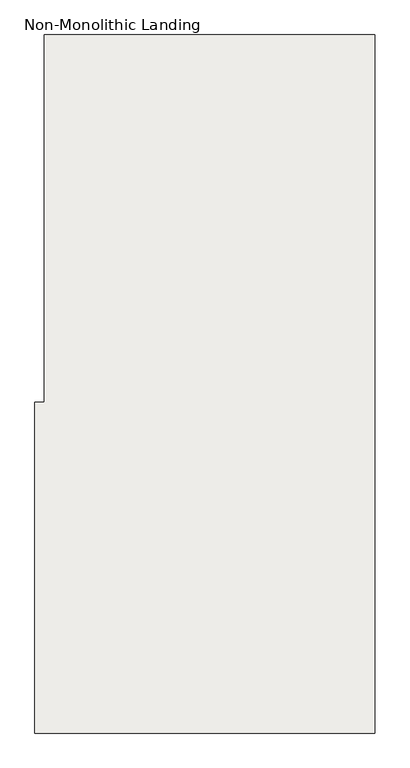
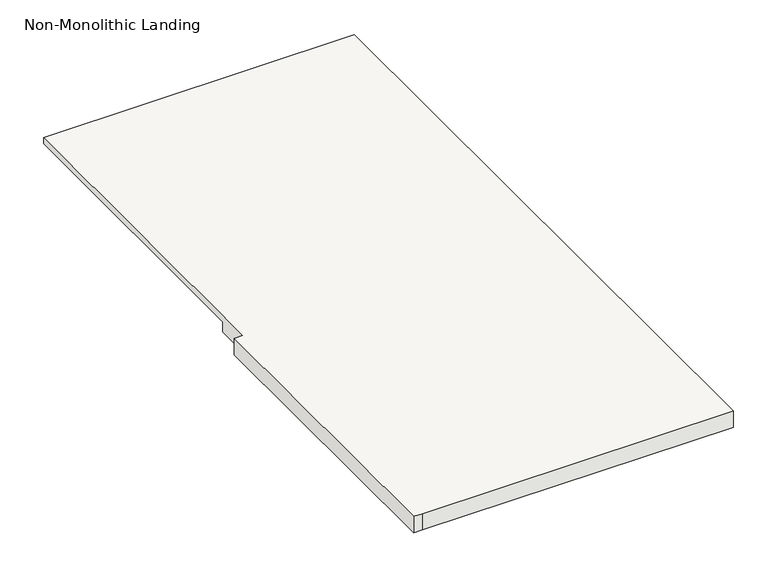
"""IFC4 building model written with IfcOpenShell, lengths in millimetres: slab geometry, Non-Monolithic Landing."""

from ifc_helpers import new_model, si_unit, origin, place, context, project, spatial, faceted_brep, source, transform, mapped, element, save


def non_monolithic_landing_f056e2ed(model_context):
    return source(origin(), model_context, "Body", "Brep", [
        faceted_brep([(923.4845537, -3822.9544725, 20783.55), (948.8845537, -3822.9544725, 20758.15), (948.8845537, -4737.3544725, 20758.15), (923.4845537, -4737.3544725, 20783.55), (923.4845537, -4838.9544725, 20802.6), (898.0845537, -4838.9544725, 20802.6), (898.0845537, -5753.3544725, 20802.6), (923.4845537, -5753.3544725, 20802.6), (1837.8845537, -5753.3544725, 20802.6), (1837.8845537, -3822.9544725, 20802.6), (923.4845537, -3822.9544725, 20802.6), (948.8845537, -4737.3544725, 20751.8), (948.8845537, -3822.9544725, 20751.8), (1837.8845537, -3822.9544725, 20751.8), (1837.8845537, -5753.3544725, 20751.8), (923.4845537, -5753.3544725, 20751.8), (898.0845537, -5753.3544725, 20751.8), (898.0845537, -4838.9544725, 20751.8), (923.4845537, -4838.9544725, 20751.8), (923.4845537, -4737.3544725, 20751.8)], [[[0, 1, 2, 3]], [[4, 5, 6, 7, 8, 9, 10]], [[11, 12, 13, 14, 15, 16, 17, 18, 19]], [[12, 11, 2, 1]], [[11, 19, 3, 2]], [[4, 10, 0, 3, 19, 18]], [[5, 4, 18, 17]], [[6, 5, 17, 16]], [[7, 6, 16, 15]], [[8, 7, 15, 14]], [[9, 8, 14, 13]], [[10, 9, 13, 12, 1, 0]]]),
    ])


if __name__ == "__main__":
    model = new_model("IFC4")
    model_context = context("Model", 3, world=origin())
    ifc_project = project(units=[si_unit("LENGTHUNIT", "METRE", prefix="MILLI")], contexts=[model_context])
    site = spatial("IfcSite", under=ifc_project)
    building = spatial("IfcBuilding", under=site)
    placement = place(None, origin())
    non_monolithic_landing_shape = non_monolithic_landing_f056e2ed(model_context)
    element("IfcSlab", 1, ObjectType="Non-Monolithic Landing", at=placement, inside=building, context=model_context, shape_type="MappedRepresentation", body=[
        mapped(non_monolithic_landing_shape, transform((0.0, 0.0, 0.0), x_axis=(1.0, 0.0, 0.0), y_axis=(0.0, 1.0, 0.0), z_axis=(0.0, 0.0, 1.0))),
    ])
    save(model, "model.ifc")
